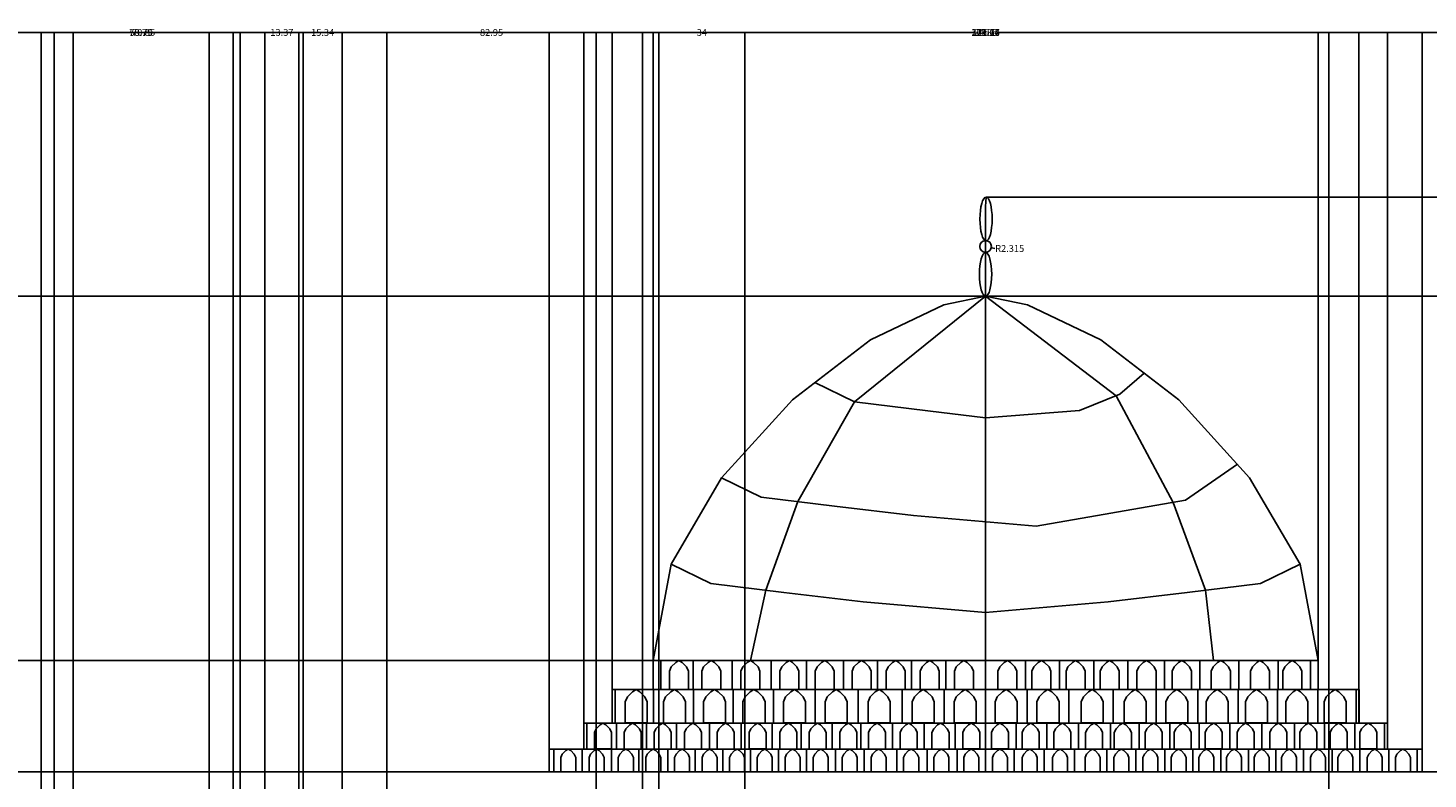
# Model space of a CAD drawing. Units: inches. Extents: x 2 to 1442, y 20 to 729.
# Tile 5 of 8: x 343 to 897, y 431 to 729. Entities that reach past the tile are written whole.
import ezdxf

# ---------------------------------------------------------------- set-up
doc = ezdxf.new("R2010")
doc.units = ezdxf.units.IN
doc.header["$MEASUREMENT"] = 0
for name, color, linetype, lineweight in [('A-ANNO-DIMS', 2, 'Continuous', 18), ('A-ELEV', 7, 'Continuous', 25), ('A-ROOF', 1, 'Continuous', 25)]:
    doc.layers.add(name, color=color, linetype=linetype, lineweight=lineweight)
doc.styles.get("Standard").update_dxf_attribs({"font": 'arial.ttf'})
doc.dimstyles.get("Standard").update_dxf_attribs({"dimtxt": 2.6875, "dimasz": 0.18, "dimexe": 0.18, "dimexo": 0.0625, "dimgap": 0.09, "dimtad": 0, "dimtih": 1, "dimtoh": 1, "dimdec": 4, "dimzin": 0, "dimdsep": 46, "dimlunit": 4, "dimtxsty": 'Standard', "dimcen": 0.09, "dimadec": 0, "dimazin": 0, "dimtfac": 1, "dimtdec": 4, "dimtofl": 0, "dimtmove": 0, "dimatfit": 3, "dimfxl": 1, "dimtolj": 1, "dimtzin": 0, "dimarcsym": 0})

# ---------------------------------------------------------------- blocks, each defined once
blk = doc.blocks.new('*D33')
at = {"layer": 'A-ANNO-DIMS', "color": 0, "lineweight": -2, "transparency": 16777216}
for p, q in [((722.06, 661.5), (1436.55, 661.5)), ((1436.37, 661.32), (1436.37, 375.85)), ((1436.37, 87.45), (1436.37, 372.92)), ((1371.19, 87.27), (1436.55, 87.27))]:
    blk.add_line(p, q, dxfattribs=at)
at = {"layer": 'A-ANNO-DIMS', "color": 0, "transparency": 16777216}
for points in [[(1436.34, 661.32), (1436.4, 661.32), (1436.37, 661.5)], [(1436.34, 87.45), (1436.4, 87.45), (1436.37, 87.27)]]:
    blk.add_solid(points, dxfattribs=at)
at = {"layer": 'Defpoints', "color": 0, "transparency": 16777216}
for p in [(722, 661.5), (1436.37, 661.5), (1371.12, 87.27)]:
    blk.add_point(p, dxfattribs=at)
at = {"layer": 'A-ANNO-DIMS', "color": 0, "transparency": 16777216, "insert": (1436.37, 374.39), "char_height": 2.688, "attachment_point": 5}
blk.add_mtext('\\A1;574.2', dxfattribs=at)
blk = doc.blocks.new('*D49')
at = {"layer": 'A-ANNO-DIMS', "color": 0, "lineweight": -2, "transparency": 16777216}
for p, q in [((353.09, 276.51), (353.09, 726.93)), ((353.27, 726.75), (383.9, 726.75)), ((423.76, 726.75), (393.14, 726.75)), ((423.94, 276.51), (423.94, 726.93))]:
    blk.add_line(p, q, dxfattribs=at)
at = {"layer": 'A-ANNO-DIMS', "color": 0, "transparency": 16777216}
for points in [[(353.27, 726.78), (353.27, 726.72), (353.09, 726.75)], [(423.76, 726.78), (423.76, 726.72), (423.94, 726.75)]]:
    blk.add_solid(points, dxfattribs=at)
at = {"layer": 'Defpoints', "color": 0, "transparency": 16777216}
for p in [(423.94, 726.75), (353.09, 276.44), (423.94, 276.44)]:
    blk.add_point(p, dxfattribs=at)
at = {"layer": 'A-ANNO-DIMS', "color": 0, "transparency": 16777216, "insert": (388.52, 726.75), "char_height": 2.688, "attachment_point": 5}
blk.add_mtext('\\A1;70.85', dxfattribs=at)
blk = doc.blocks.new('*D58')
at = {"layer": 'A-ANNO-DIMS', "color": 0, "lineweight": -2, "transparency": 16777216}
for p, q in [((347.98, 227.85), (347.98, 726.93)), ((348.16, 726.75), (382.76, 726.75)), ((426.59, 726.75), (391.99, 726.75)), ((426.77, 227.85), (426.77, 726.93))]:
    blk.add_line(p, q, dxfattribs=at)
at = {"layer": 'A-ANNO-DIMS', "color": 0, "transparency": 16777216}
for points in [[(348.16, 726.78), (348.16, 726.72), (347.98, 726.75)], [(426.59, 726.78), (426.59, 726.72), (426.77, 726.75)]]:
    blk.add_solid(points, dxfattribs=at)
at = {"layer": 'Defpoints', "color": 0, "transparency": 16777216}
for p in [(426.77, 726.75), (347.98, 227.79), (426.77, 227.79)]:
    blk.add_point(p, dxfattribs=at)
at = {"layer": 'A-ANNO-DIMS', "color": 0, "transparency": 16777216, "insert": (387.38, 726.75), "char_height": 2.688, "attachment_point": 5}
blk.add_mtext('\\A1;78.79', dxfattribs=at)
blk = doc.blocks.new('*D59')
at = {"layer": 'A-ANNO-DIMS', "color": 0, "lineweight": -2, "transparency": 16777216}
for p, q in [((360.68, 208.33), (360.68, 726.93)), ((360.86, 726.75), (382.91, 726.75)), ((414.24, 726.75), (392.18, 726.75)), ((414.42, 208.33), (414.42, 726.93))]:
    blk.add_line(p, q, dxfattribs=at)
at = {"layer": 'A-ANNO-DIMS', "color": 0, "transparency": 16777216}
for points in [[(360.86, 726.78), (360.86, 726.72), (360.68, 726.75)], [(414.24, 726.78), (414.24, 726.72), (414.42, 726.75)]]:
    blk.add_solid(points, dxfattribs=at)
at = {"layer": 'Defpoints', "color": 0, "transparency": 16777216}
for p in [(414.42, 726.75), (360.68, 208.27), (414.42, 208.27)]:
    blk.add_point(p, dxfattribs=at)
at = {"layer": 'A-ANNO-DIMS', "color": 0, "transparency": 16777216, "insert": (387.55, 726.75), "char_height": 2.688, "attachment_point": 5}
blk.add_mtext('\\A1;53.75', dxfattribs=at)
blk = doc.blocks.new('*D62')
at = {"layer": 'A-ANNO-DIMS', "color": 0, "lineweight": -2, "transparency": 16777216}
for p, q in [((436.57, 420.81), (436.57, 726.93)), ((436.75, 726.75), (438.76, 726.75)), ((449.76, 726.75), (447.75, 726.75)), ((449.94, 420.81), (449.94, 726.93))]:
    blk.add_line(p, q, dxfattribs=at)
at = {"layer": 'A-ANNO-DIMS', "color": 0, "transparency": 16777216}
for points in [[(436.75, 726.78), (436.75, 726.72), (436.57, 726.75)], [(449.76, 726.78), (449.76, 726.72), (449.94, 726.75)]]:
    blk.add_solid(points, dxfattribs=at)
at = {"layer": 'Defpoints', "color": 0, "transparency": 16777216}
for p in [(449.94, 726.75), (436.57, 420.75), (449.94, 420.75)]:
    blk.add_point(p, dxfattribs=at)
at = {"layer": 'A-ANNO-DIMS', "color": 0, "transparency": 16777216, "insert": (443.26, 726.75), "char_height": 2.688, "attachment_point": 5}
blk.add_mtext('\\A1;13.37', dxfattribs=at)
blk = doc.blocks.new('*D63')
at = {"layer": 'A-ANNO-DIMS', "color": 0, "lineweight": -2, "transparency": 16777216}
for p, q in [((451.71, 420.89), (451.71, 726.93)), ((451.89, 726.75), (454.89, 726.75)), ((466.88, 726.75), (463.88, 726.75)), ((467.06, 420.89), (467.06, 726.93))]:
    blk.add_line(p, q, dxfattribs=at)
at = {"layer": 'A-ANNO-DIMS', "color": 0, "transparency": 16777216}
for points in [[(451.89, 726.78), (451.89, 726.72), (451.71, 726.75)], [(466.88, 726.78), (466.88, 726.72), (467.06, 726.75)]]:
    blk.add_solid(points, dxfattribs=at)
at = {"layer": 'Defpoints', "color": 0, "transparency": 16777216}
for p in [(467.06, 726.75), (451.71, 420.83), (467.06, 420.83)]:
    blk.add_point(p, dxfattribs=at)
at = {"layer": 'A-ANNO-DIMS', "color": 0, "transparency": 16777216, "insert": (459.39, 726.75), "char_height": 2.688, "attachment_point": 5}
blk.add_mtext('\\A1;15.34', dxfattribs=at)
blk = doc.blocks.new('*D64')
at = {"layer": 'A-ANNO-DIMS', "color": 0, "lineweight": -2, "transparency": 16777216}
for p, q in [((590.19, 478.11), (590.19, 726.93)), ((590.37, 726.75), (716.13, 726.75)), ((853.28, 726.75), (727.52, 726.75)), ((853.46, 478.11), (853.46, 726.93))]:
    blk.add_line(p, q, dxfattribs=at)
at = {"layer": 'A-ANNO-DIMS', "color": 0, "transparency": 16777216}
for points in [[(590.37, 726.78), (590.37, 726.72), (590.19, 726.75)], [(853.28, 726.78), (853.28, 726.72), (853.46, 726.75)]]:
    blk.add_solid(points, dxfattribs=at)
at = {"layer": 'Defpoints', "color": 0, "transparency": 16777216}
for p in [(853.46, 726.75), (590.19, 478.05), (853.46, 478.05)]:
    blk.add_point(p, dxfattribs=at)
at = {"layer": 'A-ANNO-DIMS', "color": 0, "transparency": 16777216, "insert": (721.83, 726.75), "char_height": 2.688, "attachment_point": 5}
blk.add_mtext('\\A1;263.27', dxfattribs=at)
blk = doc.blocks.new('*D65')
at = {"layer": 'A-ANNO-DIMS', "color": 0, "lineweight": -2, "transparency": 16777216}
for p, q in [((549.07, 433.99), (549.07, 726.93)), ((549.25, 726.75), (717.19, 726.75)), ((894.4, 726.75), (726.46, 726.75)), ((894.58, 433.99), (894.58, 726.93))]:
    blk.add_line(p, q, dxfattribs=at)
at = {"layer": 'A-ANNO-DIMS', "color": 0, "transparency": 16777216}
for points in [[(549.25, 726.78), (549.25, 726.72), (549.07, 726.75)], [(894.4, 726.78), (894.4, 726.72), (894.58, 726.75)]]:
    blk.add_solid(points, dxfattribs=at)
at = {"layer": 'Defpoints', "color": 0, "transparency": 16777216}
for p in [(894.58, 726.75), (549.07, 433.93), (894.58, 433.93)]:
    blk.add_point(p, dxfattribs=at)
at = {"layer": 'A-ANNO-DIMS', "color": 0, "transparency": 16777216, "insert": (721.83, 726.75), "char_height": 2.688, "attachment_point": 5}
blk.add_mtext('\\A1;345.5', dxfattribs=at)
blk = doc.blocks.new('*D66')
at = {"layer": 'A-ANNO-DIMS', "color": 0, "lineweight": -2, "transparency": 16777216}
for p, q in [((562.75, 443.06), (562.75, 726.93)), ((562.93, 726.75), (716.16, 726.75)), ((880.72, 726.75), (727.49, 726.75)), ((880.9, 443.06), (880.9, 726.93))]:
    blk.add_line(p, q, dxfattribs=at)
at = {"layer": 'A-ANNO-DIMS', "color": 0, "transparency": 16777216}
for points in [[(562.93, 726.78), (562.93, 726.72), (562.75, 726.75)], [(880.72, 726.78), (880.72, 726.72), (880.9, 726.75)]]:
    blk.add_solid(points, dxfattribs=at)
at = {"layer": 'Defpoints', "color": 0, "transparency": 16777216}
for p in [(880.9, 726.75), (562.75, 442.99), (880.9, 442.99)]:
    blk.add_point(p, dxfattribs=at)
at = {"layer": 'A-ANNO-DIMS', "color": 0, "transparency": 16777216, "insert": (721.83, 726.75), "char_height": 2.688, "attachment_point": 5}
blk.add_mtext('\\A1;318.14', dxfattribs=at)
blk = doc.blocks.new('*D67')
at = {"layer": 'A-ANNO-DIMS', "color": 0, "lineweight": -2, "transparency": 16777216}
for p, q in [((574.02, 453.35), (574.02, 726.93)), ((574.2, 726.75), (717.18, 726.75)), ((869.45, 726.75), (726.47, 726.75)), ((869.63, 453.35), (869.63, 726.93))]:
    blk.add_line(p, q, dxfattribs=at)
at = {"layer": 'A-ANNO-DIMS', "color": 0, "transparency": 16777216}
for points in [[(574.2, 726.78), (574.2, 726.72), (574.02, 726.75)], [(869.45, 726.78), (869.45, 726.72), (869.63, 726.75)]]:
    blk.add_solid(points, dxfattribs=at)
at = {"layer": 'Defpoints', "color": 0, "transparency": 16777216}
for p in [(869.63, 726.75), (574.02, 453.29), (869.63, 453.29)]:
    blk.add_point(p, dxfattribs=at)
at = {"layer": 'A-ANNO-DIMS', "color": 0, "transparency": 16777216, "insert": (721.83, 726.75), "char_height": 2.688, "attachment_point": 5}
blk.add_mtext('\\A1;295.6', dxfattribs=at)
blk = doc.blocks.new('*D68')
at = {"layer": 'A-ANNO-DIMS', "color": 0, "lineweight": -2, "transparency": 16777216}
for p, q in [((721.76, 622.36), (7.1, 622.36)), ((7.28, 622.18), (7.28, 551.67)), ((7.28, 478.23), (7.28, 548.74)), ((590.13, 478.05), (7.1, 478.05))]:
    blk.add_line(p, q, dxfattribs=at)
at = {"layer": 'A-ANNO-DIMS', "color": 0, "transparency": 16777216}
for points in [[(7.25, 622.18), (7.31, 622.18), (7.28, 622.36)], [(7.25, 478.23), (7.31, 478.23), (7.28, 478.05)]]:
    blk.add_solid(points, dxfattribs=at)
at = {"layer": 'Defpoints', "color": 0, "transparency": 16777216}
for p in [(7.28, 622.36), (721.83, 622.36), (590.19, 478.05)]:
    blk.add_point(p, dxfattribs=at)
at = {"layer": 'A-ANNO-DIMS', "color": 0, "transparency": 16777216, "insert": (7.28, 550.2), "char_height": 2.688, "attachment_point": 5}
blk.add_mtext('\\A1;144.3', dxfattribs=at)
blk = doc.blocks.new('*D69')
at = {"layer": 'A-ANNO-DIMS', "color": 0, "lineweight": -2, "transparency": 16777216}
for p, q in [((590.13, 478.05), (7.1, 478.05)), ((7.28, 477.87), (7.28, 457.43)), ((7.28, 434.11), (7.28, 454.55)), ((549, 433.93), (7.1, 433.93))]:
    blk.add_line(p, q, dxfattribs=at)
at = {"layer": 'A-ANNO-DIMS', "color": 0, "transparency": 16777216}
for points in [[(7.25, 477.87), (7.31, 477.87), (7.28, 478.05)], [(7.25, 434.11), (7.31, 434.11), (7.28, 433.93)]]:
    blk.add_solid(points, dxfattribs=at)
at = {"layer": 'Defpoints', "color": 0, "transparency": 16777216}
for p in [(7.28, 478.05), (590.19, 478.05), (549.07, 433.93)]:
    blk.add_point(p, dxfattribs=at)
at = {"layer": 'A-ANNO-DIMS', "color": 0, "transparency": 16777216, "insert": (7.28, 455.99), "char_height": 2.688, "attachment_point": 5}
blk.add_mtext('\\A1;44.12', dxfattribs=at)
blk = doc.blocks.new('*D70')
at = {"layer": 'A-ANNO-DIMS', "color": 0, "lineweight": -2, "transparency": 16777216}
for p, q in [((722.06, 661.5), (1436.55, 661.5)), ((1436.37, 661.32), (1436.37, 643.39)), ((1436.37, 622.54), (1436.37, 640.47)), ((721.89, 622.36), (1436.55, 622.36))]:
    blk.add_line(p, q, dxfattribs=at)
at = {"layer": 'A-ANNO-DIMS', "color": 0, "transparency": 16777216}
for points in [[(1436.34, 661.32), (1436.4, 661.32), (1436.37, 661.5)], [(1436.34, 622.54), (1436.4, 622.54), (1436.37, 622.36)]]:
    blk.add_solid(points, dxfattribs=at)
at = {"layer": 'Defpoints', "color": 0, "transparency": 16777216}
for p in [(722, 661.5), (1436.37, 661.5), (721.83, 622.36)]:
    blk.add_point(p, dxfattribs=at)
at = {"layer": 'A-ANNO-DIMS', "color": 0, "transparency": 16777216, "insert": (1436.37, 641.93), "char_height": 2.688, "attachment_point": 5}
blk.add_mtext('\\A1;39.14', dxfattribs=at)
blk = doc.blocks.new('*D71')
at = {"layer": 'A-ANNO-DIMS', "color": 0, "lineweight": -2, "transparency": 16777216}
for p, q in [((586, 342.05), (586, 726.93)), ((586.18, 726.75), (716.12, 726.75)), ((857.47, 726.75), (727.53, 726.75)), ((857.65, 342.05), (857.65, 726.93))]:
    blk.add_line(p, q, dxfattribs=at)
at = {"layer": 'A-ANNO-DIMS', "color": 0, "transparency": 16777216}
for points in [[(586.18, 726.78), (586.18, 726.72), (586, 726.75)], [(857.47, 726.78), (857.47, 726.72), (857.65, 726.75)]]:
    blk.add_solid(points, dxfattribs=at)
at = {"layer": 'Defpoints', "color": 0, "transparency": 16777216}
for p in [(857.65, 726.75), (586, 341.99), (857.65, 341.99)]:
    blk.add_point(p, dxfattribs=at)
at = {"layer": 'A-ANNO-DIMS', "color": 0, "transparency": 16777216, "insert": (721.83, 726.75), "char_height": 2.688, "attachment_point": 5}
blk.add_mtext('\\A1;271.65', dxfattribs=at)
blk = doc.blocks.new('*D73')
at = {"layer": 'A-ANNO-DIMS', "color": 0, "lineweight": -2, "transparency": 16777216}
for p, q in [((592.5, 325.06), (592.5, 726.93)), ((592.68, 726.75), (607.49, 726.75)), ((626.32, 726.75), (611.51, 726.75)), ((626.5, 339.05), (626.5, 726.93))]:
    blk.add_line(p, q, dxfattribs=at)
at = {"layer": 'A-ANNO-DIMS', "color": 0, "transparency": 16777216}
for points in [[(592.68, 726.78), (592.68, 726.72), (592.5, 726.75)], [(626.32, 726.78), (626.32, 726.72), (626.5, 726.75)]]:
    blk.add_solid(points, dxfattribs=at)
at = {"layer": 'Defpoints', "color": 0, "transparency": 16777216}
for p in [(626.5, 726.75), (626.5, 338.99), (592.5, 325)]:
    blk.add_point(p, dxfattribs=at)
at = {"layer": 'A-ANNO-DIMS', "color": 0, "transparency": 16777216, "insert": (609.5, 726.75), "char_height": 2.688, "attachment_point": 5}
blk.add_mtext('\\A1;34', dxfattribs=at)
blk = doc.blocks.new('*D81')
at = {"layer": 'A-ANNO-DIMS', "color": 0, "lineweight": -2, "transparency": 16777216}
for p, q in [((484.77, 231.85), (484.77, 726.93)), ((484.95, 726.75), (521.61, 726.75)), ((567.54, 726.75), (530.88, 726.75)), ((567.72, 230.85), (567.72, 726.93))]:
    blk.add_line(p, q, dxfattribs=at)
at = {"layer": 'A-ANNO-DIMS', "color": 0, "transparency": 16777216}
for points in [[(484.95, 726.78), (484.95, 726.72), (484.77, 726.75)], [(567.54, 726.78), (567.54, 726.72), (567.72, 726.75)]]:
    blk.add_solid(points, dxfattribs=at)
at = {"layer": 'Defpoints', "color": 0, "transparency": 16777216}
for p in [(567.72, 726.75), (484.77, 231.79), (567.72, 230.79)]:
    blk.add_point(p, dxfattribs=at)
at = {"layer": 'A-ANNO-DIMS', "color": 0, "transparency": 16777216, "insert": (526.25, 726.75), "char_height": 2.688, "attachment_point": 5}
blk.add_mtext('\\A1;82.95', dxfattribs=at)
blk = doc.blocks.new('*D82')
at = {"layer": 'A-ANNO-DIMS', "color": 0, "lineweight": -2, "transparency": 16777216}
for p, q in [((72.53, 520.64), (72.53, 726.93)), ((72.71, 726.75), (716.28, 726.75)), ((1370.94, 726.75), (727.37, 726.75)), ((1371.12, 520.64), (1371.12, 726.93))]:
    blk.add_line(p, q, dxfattribs=at)
at = {"layer": 'A-ANNO-DIMS', "color": 0, "transparency": 16777216}
for points in [[(72.71, 726.78), (72.71, 726.72), (72.53, 726.75)], [(1370.94, 726.78), (1370.94, 726.72), (1371.12, 726.75)]]:
    blk.add_solid(points, dxfattribs=at)
at = {"layer": 'Defpoints', "color": 0, "transparency": 16777216}
for p in [(1371.12, 726.75), (72.53, 520.58), (1371.12, 520.58)]:
    blk.add_point(p, dxfattribs=at)
at = {"layer": 'A-ANNO-DIMS', "color": 0, "transparency": 16777216, "insert": (721.83, 726.75), "char_height": 2.688, "attachment_point": 5}
blk.add_mtext('\\A1;1298.6', dxfattribs=at)
blk = doc.blocks.new('*D83')
at = {"layer": 'A-ANNO-DIMS', "color": 0, "lineweight": -2, "transparency": 16777216}
for p, q in [((721.74, 642), (721.92, 642)), ((721.83, 641.91), (721.83, 642.09)), ((725.44, 641.2), (724.26, 641.46))]:
    blk.add_line(p, q, dxfattribs=at)
at = {"layer": 'A-ANNO-DIMS', "color": 0, "transparency": 16777216}
blk.add_solid([(724.27, 641.49), (724.26, 641.43), (724.09, 641.5)], dxfattribs=at)
at = {"layer": 'Defpoints', "color": 0, "transparency": 16777216}
for p in [(721.83, 642), (724.09, 641.5)]:
    blk.add_point(p, dxfattribs=at)
at = {"layer": 'A-ANNO-DIMS', "color": 0, "transparency": 16777216, "insert": (731.36, 641.2), "char_height": 2.688, "attachment_point": 5}
blk.add_mtext('\\A1;R2.315', dxfattribs=at)

msp = doc.modelspace()

# ---------------------------------------------------------------- linework, layer by layer
at = {"layer": 'A-ELEV'}
for p, q in [((590.1914, 466.5631), (590.1914, 478.0502)), ((593.2399, 478.1021), (593.2399, 466.6035)), ((606.044, 478.0589), (606.044, 466.5602)), ((621.544, 478.1021), (621.544, 466.6035)), ((636.9661, 478.0589), (636.9661, 466.5602)), ((650.9472, 478.1021), (650.9472, 466.6035)), ((665.544, 478.0589), (665.544, 466.5602)), ((679.044, 478.0589), (679.044, 466.5602)), ((692.544, 478.0589), (692.544, 466.5602)), ((706.044, 478.1021), (706.044, 466.6035)), ((737.6074, 478.1021), (737.6074, 466.6035)), ((751.1074, 478.0589), (751.1074, 466.5602)), ((764.6074, 478.0589), (764.6074, 466.5602)), ((778.1074, 478.0589), (778.1074, 466.5602)), ((792.7041, 478.1021), (792.7041, 466.6035)), ((806.6853, 478.0589), (806.6853, 466.5602)), ((822.1074, 478.1021), (822.1074, 466.6035)), ((837.6074, 478.0589), (837.6074, 466.5602)), ((850.4115, 478.1021), (850.4115, 466.6035)), ((853.4599, 466.5631), (853.4599, 478.0502)), ((574.0185, 453.2918), (574.0185, 466.5631)), ((574.0185, 466.5631), (721.8257, 466.5631)), ((575.2047, 466.6231), (575.2047, 453.3363)), ((590.3402, 466.5752), (590.3402, 453.2884)), ((606.2559, 466.6231), (606.2559, 453.3363)), ((621.8402, 466.5752), (621.8402, 453.2884)), ((637.8402, 466.6231), (637.8402, 453.3363)), ((654.3402, 466.6231), (654.3402, 453.3363)), ((671.3402, 466.6231), (671.3402, 453.3363)), ((688.8402, 466.6231), (688.8402, 453.3363)), ((705.4154, 466.6231), (705.4154, 453.3363)), ((869.6329, 466.5631), (721.8257, 466.5631)), ((738.236, 466.6231), (738.236, 453.3363)), ((754.8112, 466.6231), (754.8112, 453.3363)), ((772.3112, 466.6231), (772.3112, 453.3363)), ((789.3112, 466.6231), (789.3112, 453.3363)), ((805.8112, 466.6231), (805.8112, 453.3363)), ((821.8112, 466.5752), (821.8112, 453.2884)), ((837.3955, 466.6231), (837.3955, 453.3363)), ((853.3112, 466.5752), (853.3112, 453.2884)), ((868.4467, 466.6231), (868.4467, 453.3363)), ((869.6329, 453.2918), (869.6329, 466.5631)), ((562.7537, 442.9942), (562.7537, 453.2918)), ((562.7537, 453.2918), (721.8257, 453.2918)), ((563.9533, 453.2918), (563.9533, 443.0155)), ((575.6679, 453.2679), (575.6679, 442.9916)), ((587.6234, 453.2679), (587.6234, 442.9916)), ((599.5294, 453.2679), (599.5294, 442.9916)), ((612.4999, 453.2679), (612.4999, 442.9916)), ((625.1248, 453.2918), (625.1248, 443.0155)), ((637.3535, 453.2679), (637.3535, 442.9916)), ((648.8759, 453.2679), (648.8759, 442.9916)), ((661.0908, 453.2679), (661.0908, 442.9916)), ((672.4511, 453.2679), (672.4511, 442.9916)), ((685.0019, 453.2679), (685.0019, 442.9916)), ((697.5527, 453.2679), (697.5527, 442.9916)), ((709.7555, 453.2918), (709.7555, 443.0155)), ((880.8977, 453.2918), (721.8257, 453.2918)), ((733.8959, 453.2918), (733.8959, 443.0155)), ((746.0986, 453.2679), (746.0986, 442.9916)), ((758.6495, 453.2679), (758.6495, 442.9916)), ((771.2003, 453.2679), (771.2003, 442.9916)), ((782.5606, 453.2679), (782.5606, 442.9916)), ((794.7755, 453.2679), (794.7755, 442.9916)), ((806.2979, 453.2679), (806.2979, 442.9916)), ((818.5266, 453.2918), (818.5266, 443.0155)), ((831.1515, 453.2679), (831.1515, 442.9916)), ((844.122, 453.2679), (844.122, 442.9916)), ((856.0279, 453.2679), (856.0279, 442.9916)), ((867.9835, 453.2679), (867.9835, 442.9916)), ((879.6981, 453.2918), (879.6981, 443.0155)), ((880.8977, 442.9942), (880.8977, 453.2918)), ((549.0669, 433.9259), (549.0669, 442.9942)), ((549.0669, 442.9942), (562.7537, 442.9942)), ((550.9461, 442.9942), (550.9461, 433.9259)), ((561.2629, 442.9942), (721.8257, 442.9942)), ((562.1509, 442.9942), (562.1509, 433.9259)), ((573.7446, 442.9942), (573.7446, 433.9259)), ((584.592, 442.9942), (584.592, 433.9259)), ((596.0148, 442.9942), (596.0148, 433.9259)), ((606.9141, 442.9942), (606.9141, 433.9259)), ((617.7952, 442.9942), (617.7952, 433.9259)), ((628.7549, 442.9942), (628.7549, 433.9259)), ((639.786, 442.9942), (639.786, 433.9259)), ((650.9268, 442.9942), (650.9268, 433.9259)), ((662.3835, 442.9942), (662.3835, 433.9259)), ((673.7961, 442.9942), (673.7961, 433.9259)), ((686.6955, 442.9942), (686.6955, 433.9259)), ((698.6809, 442.9942), (698.6809, 433.9259)), ((710.505, 442.9942), (710.505, 433.9259)), ((882.3885, 442.9942), (721.8257, 442.9942)), ((733.1463, 442.9942), (733.1463, 433.9259)), ((744.9705, 442.9942), (744.9705, 433.9259)), ((756.9558, 442.9942), (756.9558, 433.9259)), ((769.8553, 442.9942), (769.8553, 433.9259)), ((781.2679, 442.9942), (781.2679, 433.9259)), ((792.7246, 442.9942), (792.7246, 433.9259)), ((803.8654, 442.9942), (803.8654, 433.9259)), ((814.8965, 442.9942), (814.8965, 433.9259)), ((825.8562, 442.9942), (825.8562, 433.9259)), ((836.7372, 442.9942), (836.7372, 433.9259)), ((847.6365, 442.9942), (847.6365, 433.9259)), ((859.0594, 442.9942), (859.0594, 433.9259)), ((869.9067, 442.9942), (869.9067, 433.9259)), ((894.5845, 442.9942), (880.8977, 442.9942)), ((881.5005, 442.9942), (881.5005, 433.9259)), ((892.7053, 442.9942), (892.7053, 433.9259)), ((894.5845, 433.9259), (894.5845, 442.9942)), ((249.3478, 433.9259), (405.1329, 433.9259)), ((405.1329, 433.9259), (431.2167, 433.9259)), ((431.2167, 433.9259), (721.8257, 433.9259)), ((1012.4347, 433.9259), (721.8257, 433.9259))]:
    msp.add_line(p, q, dxfattribs=at)
for points in [[(604.1959, 473.873), (603.4303, 475.5493), (601.6862, 477.292), (600.4188, 478.1021), (599.1515, 477.292), (597.4074, 475.5493), (596.6417, 473.873), (596.6417, 466.6063), (604.1959, 466.6063)], [(617, 473.8298), (616.2343, 475.5061), (614.4902, 477.2488), (613.2229, 478.0589), (611.9555, 477.2488), (610.2114, 475.5061), (609.4457, 473.8298), (609.4457, 466.5631), (617, 466.5631)], [(632.5, 473.873), (631.7343, 475.5493), (629.9902, 477.292), (628.7229, 478.1021), (627.4555, 477.292), (625.7114, 475.5493), (624.9457, 473.873), (624.9457, 466.6063), (632.5, 466.6063)], [(647.9221, 473.8298), (647.1564, 475.5061), (645.4123, 477.2488), (644.145, 478.0589), (642.8776, 477.2488), (641.1335, 475.5061), (640.3678, 473.8298), (640.3678, 466.5631), (647.9221, 466.5631)], [(661.9033, 473.873), (661.1376, 475.5493), (659.3935, 477.292), (658.1261, 478.1021), (656.8588, 477.292), (655.1147, 475.5493), (654.349, 473.873), (654.349, 466.6063), (661.9033, 466.6063)], [(676.5, 473.8298), (675.7343, 475.5061), (673.9902, 477.2488), (672.7229, 478.0589), (671.4555, 477.2488), (669.7114, 475.5061), (668.9457, 473.8298), (668.9457, 466.5631), (676.5, 466.5631)], [(690, 473.8298), (689.2343, 475.5061), (687.4902, 477.2488), (686.2229, 478.0589), (684.9555, 477.2488), (683.2114, 475.5061), (682.4457, 473.8298), (682.4457, 466.5631), (690, 466.5631)], [(703.5, 473.8298), (702.7343, 475.5061), (700.9902, 477.2488), (699.7229, 478.0589), (698.4555, 477.2488), (696.7114, 475.5061), (695.9457, 473.8298), (695.9457, 466.5631), (703.5, 466.5631)], [(717, 473.873), (716.2343, 475.5493), (714.4902, 477.292), (713.2229, 478.1021), (711.9555, 477.292), (710.2114, 475.5493), (709.4457, 473.873), (709.4457, 466.6063), (717, 466.6063)], [(726.6514, 473.873), (727.4171, 475.5493), (729.1611, 477.292), (730.4285, 478.1021), (731.6959, 477.292), (733.44, 475.5493), (734.2056, 473.873), (734.2056, 466.6063), (726.6514, 466.6063)], [(740.1514, 473.8298), (740.9171, 475.5061), (742.6611, 477.2488), (743.9285, 478.0589), (745.1959, 477.2488), (746.94, 475.5061), (747.7056, 473.8298), (747.7056, 466.5631), (740.1514, 466.5631)], [(753.6514, 473.8298), (754.4171, 475.5061), (756.1611, 477.2488), (757.4285, 478.0589), (758.6959, 477.2488), (760.44, 475.5061), (761.2056, 473.8298), (761.2056, 466.5631), (753.6514, 466.5631)], [(767.1514, 473.8298), (767.9171, 475.5061), (769.6611, 477.2488), (770.9285, 478.0589), (772.1959, 477.2488), (773.94, 475.5061), (774.7056, 473.8298), (774.7056, 466.5631), (767.1514, 466.5631)], [(781.7481, 473.873), (782.5138, 475.5493), (784.2579, 477.292), (785.5252, 478.1021), (786.7926, 477.292), (788.5367, 475.5493), (789.3024, 473.873), (789.3024, 466.6063), (781.7481, 466.6063)], [(795.7293, 473.8298), (796.495, 475.5061), (798.2391, 477.2488), (799.5064, 478.0589), (800.7738, 477.2488), (802.5179, 475.5061), (803.2835, 473.8298), (803.2835, 466.5631), (795.7293, 466.5631)], [(811.1514, 473.873), (811.9171, 475.5493), (813.6611, 477.292), (814.9285, 478.1021), (816.1959, 477.292), (817.94, 475.5493), (818.7056, 473.873), (818.7056, 466.6063), (811.1514, 466.6063)], [(826.6514, 473.8298), (827.4171, 475.5061), (829.1611, 477.2488), (830.4285, 478.0589), (831.6959, 477.2488), (833.44, 475.5061), (834.2056, 473.8298), (834.2056, 466.5631), (826.6514, 466.5631)], [(839.4554, 473.873), (840.2211, 475.5493), (841.9652, 477.292), (843.2326, 478.1021), (844.4999, 477.292), (846.244, 475.5493), (847.0097, 473.873), (847.0097, 466.6063), (839.4554, 466.6063)], [(587.8645, 461.7363), (586.9798, 463.6733), (584.9644, 465.687), (583.5, 466.6231), (582.0356, 465.687), (580.0202, 463.6733), (579.1355, 461.7363), (579.1355, 453.3397), (587.8645, 453.3397)], [(603, 461.6884), (602.1153, 463.6254), (600.0999, 465.6391), (598.6355, 466.5752), (597.1711, 465.6391), (595.1557, 463.6254), (594.271, 461.6884), (594.271, 453.2918), (603, 453.2918)], [(618.9157, 461.7363), (618.0309, 463.6733), (616.0156, 465.687), (614.5511, 466.6231), (613.0867, 465.687), (611.0714, 463.6733), (610.1866, 461.7363), (610.1866, 453.3397), (618.9157, 453.3397)], [(634.5, 461.6884), (633.6153, 463.6254), (631.5999, 465.6391), (630.1355, 466.5752), (628.6711, 465.6391), (626.6557, 463.6254), (625.771, 461.6884), (625.771, 453.2918), (634.5, 453.2918)], [(650.5, 461.7363), (649.6153, 463.6733), (647.5999, 465.687), (646.1355, 466.6231), (644.6711, 465.687), (642.6557, 463.6733), (641.771, 461.7363), (641.771, 453.3397), (650.5, 453.3397)], [(667, 461.7363), (666.1153, 463.6733), (664.0999, 465.687), (662.6355, 466.6231), (661.1711, 465.687), (659.1557, 463.6733), (658.271, 461.7363), (658.271, 453.3397), (667, 453.3397)], [(684, 461.7363), (683.1153, 463.6733), (681.0999, 465.687), (679.6355, 466.6231), (678.1711, 465.687), (676.1557, 463.6733), (675.271, 461.7363), (675.271, 453.3397), (684, 453.3397)], [(701.5, 461.7363), (700.6153, 463.6733), (698.5999, 465.687), (697.1355, 466.6231), (695.6711, 465.687), (693.6557, 463.6733), (692.771, 461.7363), (692.771, 453.3397), (701.5, 453.3397)], [(718.0752, 461.7363), (717.1904, 463.6733), (715.1751, 465.687), (713.7107, 466.6231), (712.2462, 465.687), (710.2309, 463.6733), (709.3462, 461.7363), (709.3462, 453.3397), (718.0752, 453.3397)], [(725.5762, 461.7363), (726.4609, 463.6733), (728.4763, 465.687), (729.9407, 466.6231), (731.4051, 465.687), (733.4205, 463.6733), (734.3052, 461.7363), (734.3052, 453.3397), (725.5762, 453.3397)], [(742.1514, 461.7363), (743.0361, 463.6733), (745.0514, 465.687), (746.5159, 466.6231), (747.9803, 465.687), (749.9956, 463.6733), (750.8804, 461.7363), (750.8804, 453.3397), (742.1514, 453.3397)], [(759.6514, 461.7363), (760.5361, 463.6733), (762.5514, 465.687), (764.0159, 466.6231), (765.4803, 465.687), (767.4956, 463.6733), (768.3804, 461.7363), (768.3804, 453.3397), (759.6514, 453.3397)], [(776.6514, 461.7363), (777.5361, 463.6733), (779.5514, 465.687), (781.0159, 466.6231), (782.4803, 465.687), (784.4956, 463.6733), (785.3804, 461.7363), (785.3804, 453.3397), (776.6514, 453.3397)], [(793.1514, 461.7363), (794.0361, 463.6733), (796.0514, 465.687), (797.5159, 466.6231), (798.9803, 465.687), (800.9956, 463.6733), (801.8804, 461.7363), (801.8804, 453.3397), (793.1514, 453.3397)], [(809.1514, 461.6884), (810.0361, 463.6254), (812.0514, 465.6391), (813.5159, 466.5752), (814.9803, 465.6391), (816.9956, 463.6254), (817.8804, 461.6884), (817.8804, 453.2918), (809.1514, 453.2918)], [(824.7357, 461.7363), (825.6205, 463.6733), (827.6358, 465.687), (829.1002, 466.6231), (830.5647, 465.687), (832.58, 463.6733), (833.4647, 461.7363), (833.4647, 453.3397), (824.7357, 453.3397)], [(840.6514, 461.6884), (841.5361, 463.6254), (843.5514, 465.6391), (845.0159, 466.5752), (846.4803, 465.6391), (848.4956, 463.6254), (849.3804, 461.6884), (849.3804, 453.2918), (840.6514, 453.2918)], [(855.7869, 461.7363), (856.6716, 463.6733), (858.6869, 465.687), (860.1514, 466.6231), (861.6158, 465.687), (863.6311, 463.6733), (864.5159, 461.7363), (864.5159, 453.3397), (855.7869, 453.3397)], [(573.7446, 449.5122), (573.0603, 451.0103), (571.5017, 452.5678), (570.369, 453.2918), (569.2364, 452.5678), (567.6777, 451.0103), (566.9934, 449.5122), (566.9934, 443.018), (573.7446, 443.018)], [(585.4593, 449.4884), (584.775, 450.9865), (583.2163, 452.5439), (582.0837, 453.2679), (580.951, 452.5439), (579.3923, 450.9865), (578.7081, 449.4884), (578.7081, 442.9942), (585.4593, 442.9942)], [(597.4148, 449.4884), (596.7305, 450.9865), (595.1718, 452.5439), (594.0392, 453.2679), (592.9066, 452.5439), (591.3479, 450.9865), (590.6636, 449.4884), (590.6636, 442.9942), (597.4148, 442.9942)], [(609.3208, 449.4884), (608.6365, 450.9865), (607.0778, 452.5439), (605.9452, 453.2679), (604.8125, 452.5439), (603.2538, 450.9865), (602.5695, 449.4884), (602.5695, 442.9942), (609.3208, 442.9942)], [(622.2913, 449.4884), (621.607, 450.9865), (620.0483, 452.5439), (618.9157, 453.2679), (617.783, 452.5439), (616.2243, 450.9865), (615.54, 449.4884), (615.54, 442.9942), (622.2913, 442.9942)], [(634.9162, 449.5122), (634.2319, 451.0103), (632.6732, 452.5678), (631.5406, 453.2918), (630.408, 452.5678), (628.8493, 451.0103), (628.165, 449.5122), (628.165, 443.018), (634.9162, 443.018)], [(647.1449, 449.4884), (646.4606, 450.9865), (644.9019, 452.5439), (643.7693, 453.2679), (642.6367, 452.5439), (641.078, 450.9865), (640.3937, 449.4884), (640.3937, 442.9942), (647.1449, 442.9942)], [(658.6673, 449.4884), (657.983, 450.9865), (656.4243, 452.5439), (655.2917, 453.2679), (654.1591, 452.5439), (652.6004, 450.9865), (651.9161, 449.4884), (651.9161, 442.9942), (658.6673, 442.9942)], [(670.8822, 449.4884), (670.1979, 450.9865), (668.6392, 452.5439), (667.5066, 453.2679), (666.3739, 452.5439), (664.8153, 450.9865), (664.131, 449.4884), (664.131, 442.9942), (670.8822, 442.9942)], [(682.2424, 449.4884), (681.5582, 450.9865), (679.9995, 452.5439), (678.8668, 453.2679), (677.7342, 452.5439), (676.1755, 450.9865), (675.4912, 449.4884), (675.4912, 442.9942), (682.2424, 442.9942)], [(694.7933, 449.4884), (694.109, 450.9865), (692.5503, 452.5439), (691.4177, 453.2679), (690.285, 452.5439), (688.7264, 450.9865), (688.0421, 449.4884), (688.0421, 442.9942), (694.7933, 442.9942)], [(707.3441, 449.4884), (706.6598, 450.9865), (705.1011, 452.5439), (703.9685, 453.2679), (702.8359, 452.5439), (701.2772, 450.9865), (700.5929, 449.4884), (700.5929, 442.9942), (707.3441, 442.9942)], [(719.5469, 449.5122), (718.8626, 451.0103), (717.3039, 452.5678), (716.1713, 453.2918), (715.0386, 452.5678), (713.48, 451.0103), (712.7957, 449.5122), (712.7957, 443.018), (719.5469, 443.018)], [(724.1045, 449.5122), (724.7888, 451.0103), (726.3475, 452.5678), (727.4801, 453.2918), (728.6127, 452.5678), (730.1714, 451.0103), (730.8557, 449.5122), (730.8557, 443.018), (724.1045, 443.018)], [(736.3073, 449.4884), (736.9915, 450.9865), (738.5502, 452.5439), (739.6829, 453.2679), (740.8155, 452.5439), (742.3742, 450.9865), (743.0585, 449.4884), (743.0585, 442.9942), (736.3073, 442.9942)], [(748.8581, 449.4884), (749.5424, 450.9865), (751.1011, 452.5439), (752.2337, 453.2679), (753.3663, 452.5439), (754.925, 450.9865), (755.6093, 449.4884), (755.6093, 442.9942), (748.8581, 442.9942)], [(761.4089, 449.4884), (762.0932, 450.9865), (763.6519, 452.5439), (764.7845, 453.2679), (765.9172, 452.5439), (767.4759, 450.9865), (768.1601, 449.4884), (768.1601, 442.9942), (761.4089, 442.9942)], [(772.7692, 449.4884), (773.4535, 450.9865), (775.0122, 452.5439), (776.1448, 453.2679), (777.2774, 452.5439), (778.8361, 450.9865), (779.5204, 449.4884), (779.5204, 442.9942), (772.7692, 442.9942)], [(784.9841, 449.4884), (785.6684, 450.9865), (787.227, 452.5439), (788.3597, 453.2679), (789.4923, 452.5439), (791.051, 450.9865), (791.7353, 449.4884), (791.7353, 442.9942), (784.9841, 442.9942)], [(796.5065, 449.4884), (797.1908, 450.9865), (798.7494, 452.5439), (799.8821, 453.2679), (801.0147, 452.5439), (802.5734, 450.9865), (803.2577, 449.4884), (803.2577, 442.9942), (796.5065, 442.9942)], [(808.7352, 449.5122), (809.4195, 451.0103), (810.9781, 452.5678), (812.1108, 453.2918), (813.2434, 452.5678), (814.8021, 451.0103), (815.4864, 449.5122), (815.4864, 443.018), (808.7352, 443.018)], [(821.3601, 449.4884), (822.0444, 450.9865), (823.6031, 452.5439), (824.7357, 453.2679), (825.8684, 452.5439), (827.427, 450.9865), (828.1113, 449.4884), (828.1113, 442.9942), (821.3601, 442.9942)], [(834.3306, 449.4884), (835.0149, 450.9865), (836.5736, 452.5439), (837.7062, 453.2679), (838.8389, 452.5439), (840.3975, 450.9865), (841.0818, 449.4884), (841.0818, 442.9942), (834.3306, 442.9942)], [(846.2366, 449.4884), (846.9208, 450.9865), (848.4795, 452.5439), (849.6122, 453.2679), (850.7448, 452.5439), (852.3035, 450.9865), (852.9878, 449.4884), (852.9878, 442.9942), (846.2366, 442.9942)], [(858.1921, 449.4884), (858.8764, 450.9865), (860.4351, 452.5439), (861.5677, 453.2679), (862.7003, 452.5439), (864.259, 450.9865), (864.9433, 449.4884), (864.9433, 442.9942), (858.1921, 442.9942)], [(869.9067, 449.5122), (870.591, 451.0103), (872.1497, 452.5678), (873.2823, 453.2918), (874.415, 452.5678), (875.9737, 451.0103), (876.658, 449.5122), (876.658, 443.018), (869.9067, 443.018)], [(559.5864, 439.659), (558.9826, 440.981), (557.6071, 442.3553), (556.6076, 442.9942), (555.6082, 442.3553), (554.2327, 440.981), (553.6289, 439.659), (553.6289, 433.9282), (559.5864, 433.9282)], [(570.7913, 439.659), (570.1874, 440.981), (568.812, 442.3553), (567.8125, 442.9942), (566.813, 442.3553), (565.4375, 440.981), (564.8337, 439.659), (564.8337, 433.9282), (570.7913, 433.9282)], [(582.385, 439.659), (581.7811, 440.981), (580.4057, 442.3553), (579.4062, 442.9942), (578.4067, 442.3553), (577.0313, 440.981), (576.4274, 439.659), (576.4274, 433.9282), (582.385, 433.9282)], [(593.2323, 439.659), (592.6285, 440.981), (591.253, 442.3553), (590.2535, 442.9942), (589.2541, 442.3553), (587.8786, 440.981), (587.2748, 439.659), (587.2748, 433.9282), (593.2323, 433.9282)], [(604.6552, 439.659), (604.0513, 440.981), (602.6759, 442.3553), (601.6764, 442.9942), (600.6769, 442.3553), (599.3015, 440.981), (598.6976, 439.659), (598.6976, 433.9282), (604.6552, 433.9282)], [(615.5545, 439.659), (614.9507, 440.981), (613.5752, 442.3553), (612.5757, 442.9942), (611.5762, 442.3553), (610.2008, 440.981), (609.5969, 439.659), (609.5969, 433.9282), (615.5545, 433.9282)], [(626.4356, 439.659), (625.8317, 440.981), (624.4563, 442.3553), (623.4568, 442.9942), (622.4573, 442.3553), (621.0818, 440.981), (620.478, 439.659), (620.478, 433.9282), (626.4356, 433.9282)], [(637.3952, 439.659), (636.7914, 440.981), (635.4159, 442.3553), (634.4165, 442.9942), (633.417, 442.3553), (632.0415, 440.981), (631.4377, 439.659), (631.4377, 433.9282), (637.3952, 433.9282)], [(648.4263, 439.659), (647.8225, 440.981), (646.447, 442.3553), (645.4475, 442.9942), (644.448, 442.3553), (643.0726, 440.981), (642.4687, 439.659), (642.4687, 433.9282), (648.4263, 433.9282)], [(659.5671, 439.659), (658.9633, 440.981), (657.5879, 442.3553), (656.5884, 442.9942), (655.5889, 442.3553), (654.2134, 440.981), (653.6096, 439.659), (653.6096, 433.9282), (659.5671, 433.9282)], [(671.0239, 439.659), (670.42, 440.981), (669.0446, 442.3553), (668.0451, 442.9942), (667.0456, 442.3553), (665.6701, 440.981), (665.0663, 439.659), (665.0663, 433.9282), (671.0239, 433.9282)], [(682.4364, 439.659), (681.8326, 440.981), (680.4571, 442.3553), (679.4577, 442.9942), (678.4582, 442.3553), (677.0827, 440.981), (676.4789, 439.659), (676.4789, 433.9282), (682.4364, 433.9282)], [(695.3359, 439.659), (694.732, 440.981), (693.3566, 442.3553), (692.3571, 442.9942), (691.3576, 442.3553), (689.9821, 440.981), (689.3783, 439.659), (689.3783, 433.9282), (695.3359, 433.9282)], [(707.3213, 439.659), (706.7174, 440.981), (705.342, 442.3553), (704.3425, 442.9942), (703.343, 442.3553), (701.9675, 440.981), (701.3637, 439.659), (701.3637, 433.9282), (707.3213, 433.9282)], [(719.1454, 439.659), (718.5415, 440.981), (717.1661, 442.3553), (716.1666, 442.9942), (715.1671, 442.3553), (713.7917, 440.981), (713.1878, 439.659), (713.1878, 433.9282), (719.1454, 433.9282)], [(724.506, 439.659), (725.1098, 440.981), (726.4853, 442.3553), (727.4848, 442.9942), (728.4843, 442.3553), (729.8597, 440.981), (730.4636, 439.659), (730.4636, 433.9282), (724.506, 433.9282)], [(736.3301, 439.659), (736.934, 440.981), (738.3094, 442.3553), (739.3089, 442.9942), (740.3084, 442.3553), (741.6839, 440.981), (742.2877, 439.659), (742.2877, 433.9282), (736.3301, 433.9282)], [(748.3155, 439.659), (748.9193, 440.981), (750.2948, 442.3553), (751.2943, 442.9942), (752.2938, 442.3553), (753.6692, 440.981), (754.2731, 439.659), (754.2731, 433.9282), (748.3155, 433.9282)], [(761.2149, 439.659), (761.8188, 440.981), (763.1942, 442.3553), (764.1937, 442.9942), (765.1932, 442.3553), (766.5687, 440.981), (767.1725, 439.659), (767.1725, 433.9282), (761.2149, 433.9282)], [(772.6275, 439.659), (773.2313, 440.981), (774.6068, 442.3553), (775.6063, 442.9942), (776.6058, 442.3553), (777.9812, 440.981), (778.5851, 439.659), (778.5851, 433.9282), (772.6275, 433.9282)], [(784.0842, 439.659), (784.6881, 440.981), (786.0635, 442.3553), (787.063, 442.9942), (788.0625, 442.3553), (789.438, 440.981), (790.0418, 439.659), (790.0418, 433.9282), (784.0842, 433.9282)], [(795.2251, 439.659), (795.8289, 440.981), (797.2044, 442.3553), (798.2038, 442.9942), (799.2033, 442.3553), (800.5788, 440.981), (801.1826, 439.659), (801.1826, 433.9282), (795.2251, 433.9282)], [(806.2561, 439.659), (806.86, 440.981), (808.2354, 442.3553), (809.2349, 442.9942), (810.2344, 442.3553), (811.6099, 440.981), (812.2137, 439.659), (812.2137, 433.9282), (806.2561, 433.9282)], [(817.2158, 439.659), (817.8197, 440.981), (819.1951, 442.3553), (820.1946, 442.9942), (821.1941, 442.3553), (822.5695, 440.981), (823.1734, 439.659), (823.1734, 433.9282), (817.2158, 433.9282)], [(828.0969, 439.659), (828.7007, 440.981), (830.0762, 442.3553), (831.0757, 442.9942), (832.0751, 442.3553), (833.4506, 440.981), (834.0544, 439.659), (834.0544, 433.9282), (828.0969, 433.9282)], [(838.9962, 439.659), (839.6, 440.981), (840.9755, 442.3553), (841.975, 442.9942), (842.9745, 442.3553), (844.3499, 440.981), (844.9538, 439.659), (844.9538, 433.9282), (838.9962, 433.9282)], [(850.419, 439.659), (851.0229, 440.981), (852.3983, 442.3553), (853.3978, 442.9942), (854.3973, 442.3553), (855.7728, 440.981), (856.3766, 439.659), (856.3766, 433.9282), (850.419, 433.9282)], [(861.2664, 439.659), (861.8702, 440.981), (863.2457, 442.3553), (864.2452, 442.9942), (865.2447, 442.3553), (866.6201, 440.981), (867.224, 439.659), (867.224, 433.9282), (861.2664, 433.9282)], [(872.8601, 439.659), (873.464, 440.981), (874.8394, 442.3553), (875.8389, 442.9942), (876.8384, 442.3553), (878.2138, 440.981), (878.8177, 439.659), (878.8177, 433.9282), (872.8601, 433.9282)], [(884.0649, 439.659), (884.6688, 440.981), (886.0442, 442.3553), (887.0437, 442.9942), (888.0432, 442.3553), (889.4187, 440.981), (890.0225, 439.659), (890.0225, 433.9282), (884.0649, 433.9282)]]:
    msp.add_lwpolyline(points, close=True, dxfattribs=at)
at = {"layer": 'A-ROOF'}
for p, q in [((721.8257, 657.801), (722.0388, 661.4989)), ((721.8257, 433.9259), (721.8257, 657.801)), ((590.1914, 478.0502), (721.8257, 478.0502)), ((853.4599, 478.0502), (721.8257, 478.0502))]:
    msp.add_line(p, q, dxfattribs=at)
for points in [[(590.1914, 478.0502), (597.35, 516.2436), (617.313, 550.4384), (645.3562, 581.3088), (676.2513, 605.0552), (705.2452, 618.8281), (721.8257, 622.3576)], [(721.8257, 622.3576), (669.9145, 580.4122), (647.463, 540.9448), (634.8626, 505.8614), (628.7229, 478.1021)], [(853.4599, 478.0502), (846.3014, 516.2436), (826.3384, 550.4384), (798.2951, 581.3088), (767.4001, 605.0552), (738.4062, 618.8281), (721.8257, 622.3576)], [(721.8257, 622.3576), (773.4577, 582.8734), (796.0625, 540.6407), (808.8945, 505.8742), (812, 478.0502)], [(654.2645, 588.1558), (669.9145, 580.4122), (698.9145, 576.9122), (721.8257, 574.1471), (721.8257, 574.1471)], [(721.8257, 574.1471), (759, 577), (775, 583.5), (784.5536, 591.8707)], [(741.7887, 531.1948), (801, 541.5), (821.4968, 555.7681)], [(617.313, 550.4384), (632.963, 542.6948), (661.963, 539.1948), (693.3081, 535.4118), (741.7887, 531.1948)], [(597.35, 516.2436), (613, 508.5), (642, 505), (673.3452, 501.217), (721.8257, 497)], [(846.3014, 516.2436), (830.6514, 508.5), (801.6514, 505), (770.3062, 501.217), (721.8257, 497)]]:
    msp.add_lwpolyline(points, dxfattribs=at)
for start, end in [(90, 270), (270, 90)]:
    msp.add_arc((721.8257, 642), 2.3151, start, end, dxfattribs=at)
for centre in [(722, 652.8576), (721.8257, 631)]:
    msp.add_ellipse(centre, major_axis=(0, 8.6424), ratio=0.27917915, dxfattribs=at)

# ---------------------------------------------------------------- dimensions: what is measured, and where the dimension line sits
at = {"layer": 'A-ANNO-DIMS'}
for base, p1, p2, override, picture, middle in [((1371.1242, 726.75), (72.5272, 520.5823), (1371.1242, 520.5823), {"dimdec": 1, "dimlfac": 1, "dimrnd": 0, "dimzin": 0, "dimdsep": 46, "dimlunit": 2}, '*D82', (721.8257, 726.75)), ((426.7688, 726.75), (347.9824, 227.7901), (426.7688, 227.7901), {"dimdec": 2, "dimlfac": 1, "dimrnd": 0, "dimzin": 0, "dimdsep": 46, "dimlunit": 2}, '*D58', (387.3756, 726.75)), ((423.9427, 726.75), (353.095, 276.443), (423.9427, 276.443), {"dimdec": 2, "dimlfac": 1, "dimrnd": 0, "dimzin": 0, "dimdsep": 46, "dimlunit": 2}, '*D49', (388.5188, 726.75)), ((414.4218, 726.75), (360.6755, 208.2722), (414.4218, 208.2722), {"dimdec": 2, "dimlfac": 1, "dimrnd": 0, "dimzin": 0, "dimdsep": 46, "dimlunit": 2}, '*D59', (387.5486, 726.75)), ((449.94, 726.75), (436.5711, 420.7472), (449.94, 420.7472), {"dimdec": 2, "dimlfac": 1, "dimrnd": 0, "dimzin": 0, "dimdsep": 46, "dimlunit": 2}, '*D62', (443.2556, 726.75)), ((467.0558, 726.75), (451.7146, 420.8293), (467.0558, 420.8293), {"dimdec": 2, "dimlfac": 1, "dimrnd": 0, "dimzin": 0, "dimdsep": 46, "dimlunit": 2}, '*D63', (459.3852, 726.75)), ((567.72, 726.75), (484.7727, 231.7901), (567.72, 230.7901), {"dimdec": 2, "dimlfac": 1, "dimrnd": 0, "dimzin": 0, "dimdsep": 46, "dimlunit": 2}, '*D81', (526.2463, 726.75)), ((894.5845, 726.75), (549.0669, 433.9259), (894.5845, 433.9259), {"dimdec": 1, "dimlfac": 1, "dimrnd": 0, "dimzin": 0, "dimdsep": 46, "dimlunit": 2}, '*D65', (721.8257, 726.75)), ((880.8977, 726.75), (562.7537, 442.9942), (880.8977, 442.9942), {"dimdec": 2, "dimlfac": 1, "dimrnd": 0, "dimzin": 0, "dimdsep": 46, "dimlunit": 2}, '*D66', (721.8257, 726.75)), ((869.6329, 726.75), (574.0185, 453.2918), (869.6329, 453.2918), {"dimdec": 1, "dimlfac": 1, "dimrnd": 0, "dimzin": 0, "dimdsep": 46, "dimlunit": 2}, '*D67', (721.8257, 726.75)), ((857.6514, 726.75), (586, 341.9894), (857.6514, 341.9894), {"dimdec": 2, "dimlfac": 1, "dimrnd": 0, "dimzin": 0, "dimdsep": 46, "dimlunit": 2}, '*D71', (721.8257, 726.75)), ((853.4599, 726.75), (590.1914, 478.0502), (853.4599, 478.0502), {"dimdec": 2, "dimlfac": 1, "dimrnd": 0, "dimzin": 0, "dimdsep": 46, "dimlunit": 2}, '*D64', (721.8257, 726.75)), ((626.5, 726.75), (592.5, 325), (626.5, 338.9894), {"dimdec": 0, "dimlfac": 1, "dimrnd": 0, "dimzin": 0, "dimdsep": 46, "dimlunit": 2}, '*D73', (609.5, 726.75))]:
    dim = msp.add_linear_dim(base=base, p1=p1, p2=p2, dimstyle='Standard', override=override, dxfattribs=at)
    dim.commit()
    dim.dimension.update_dxf_attribs({"geometry": picture, "text_midpoint": middle})
for base, p1, p2, override, picture, middle in [((1436.3742, 661.5), (721.8257, 622.3576), (722, 661.5), {"dimdec": 2, "dimlfac": 1, "dimrnd": 0, "dimzin": 0, "dimdsep": 46, "dimlunit": 2}, '*D70', (1436.3742, 641.9288)), ((1436.3742, 661.5), (1371.1242, 87.2714), (722, 661.5), {"dimdec": 1, "dimlfac": 1, "dimrnd": 0, "dimzin": 0, "dimdsep": 46, "dimlunit": 2}, '*D33', (1436.3742, 374.3857)), ((7.2772, 622.3576), (590.1914, 478.0502), (721.8257, 622.3576), {"dimdec": 1, "dimlfac": 1, "dimrnd": 0, "dimzin": 0, "dimdsep": 46, "dimlunit": 2}, '*D68', (7.2772, 550.2039)), ((7.2772, 478.0502), (549.0669, 433.9259), (590.1914, 478.0502), {"dimdec": 2, "dimlfac": 1, "dimrnd": 0, "dimzin": 0, "dimdsep": 46, "dimlunit": 2}, '*D69', (7.2772, 455.9881))]:
    dim = msp.add_linear_dim(base=base, p1=p1, p2=p2, angle=90, dimstyle='Standard', override=override, dxfattribs=at)
    dim.commit()
    dim.dimension.update_dxf_attribs({"geometry": picture, "text_midpoint": middle})
dim = msp.add_radius_dim(center=(721.8257, 642), mpoint=(724.0867, 641.5029), dimstyle='Standard', override={"dimdec": 3, "dimlfac": 1, "dimrnd": 0, "dimzin": 0, "dimdsep": 46, "dimlunit": 2}, dxfattribs=at)
dim.commit()
dim.dimension.update_dxf_attribs({"geometry": '*D83', "text_midpoint": (725.4434, 641.2047), "dimtype": 164})

doc.saveas('drawing.dxf')
